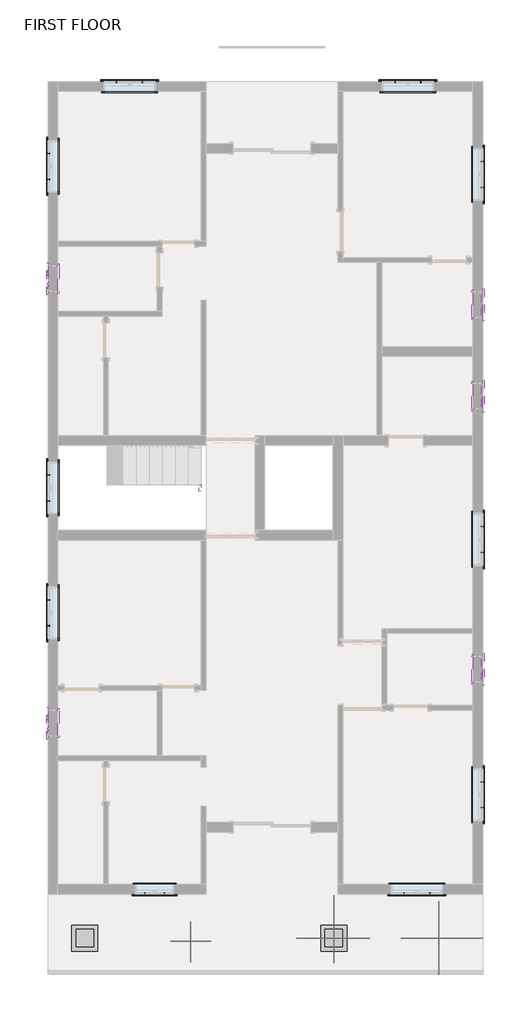
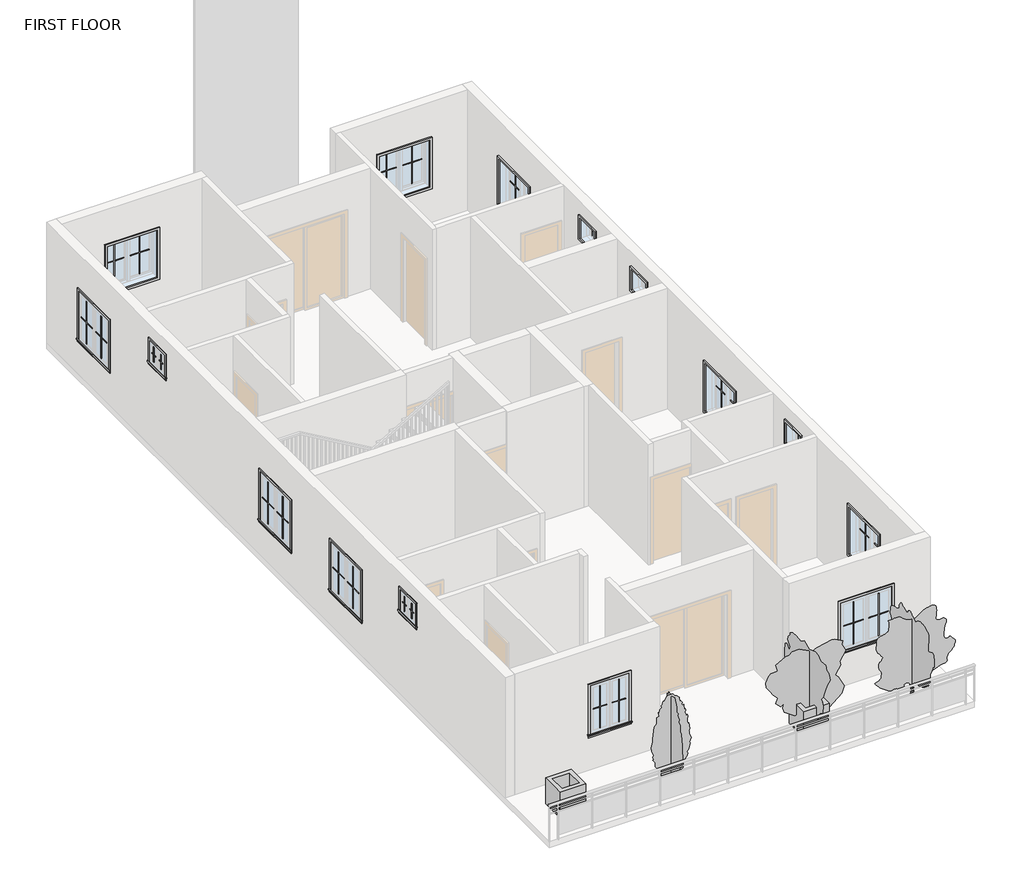
# One storey, part 4 of 4: 60 proxies, 5 geographic elements, 1 railing.
"""IFC4 building model written with IfcOpenShell, lengths in millimetres."""

from ifc_helpers import new_model, si_unit, frame, origin, place, context, project, spatial, polyline, outline, extrude, transform, mapped, element, save
from components import muntin_pattern_2x2_muntin_pattern_2x2_4dfeb3f3, muntin_pattern_2x2_muntin_pattern_2x2_e852a7e4, muntin_pattern_2x2_muntin_pattern_2x2_1acec82f, muntin_pattern_2x2_muntin_pattern_2x2_43d02eee, muntin_pattern_2x2_muntin_pattern_2x2_653c8599, muntin_pattern_2x2_muntin_pattern_2x2_c179cf80, trim_window_exterior_flat_with_sill_7cfdd449, trim_window_exterior_flat_with_sill_e4b28ec3, trim_window_exterior_flat_with_sill_e6f34eb5, trim_window_interior_flat_picture_frame_f1e0b15b, trim_window_interior_flat_picture_frame_39ff4276, trim_window_interior_flat_picture_frame_9a74d23d, planter_2_x2_5b049b04, rpc_tree_conifer_chinese_juniper_7_2_1b9786cd, rpc_tree_fall_american_beech_20_7ed35302, rpc_tree_fall_service_berry_25_c2e4521a

model = new_model("IFC4")

# Units and contexts
model_context = context("Model", 3, world=origin())
ifc_project = project(units=[si_unit("LENGTHUNIT", "METRE", prefix="MILLI")], contexts=[model_context])

# Site, building, storey
site = spatial("IfcSite", under=ifc_project)
building = spatial("IfcBuilding", under=site)
storey = spatial("IfcBuildingStorey", under=building, Name="FIRST FLOOR", Elevation=3200.4)

# Proxies
placement = place(None, origin())
muntin_pattern_2x2_muntin_pattern_2x2_shape = muntin_pattern_2x2_muntin_pattern_2x2_4dfeb3f3(model_context)
element("IfcBuildingElementProxy", 1, Name="Muntin Pattern_2x2 : Muntin Pattern_2x2", ObjectType="Muntin Pattern_2x2 : Muntin Pattern_2x2", at=placement, inside=storey, context=model_context, shape_type="MappedRepresentation", body=[
    mapped(muntin_pattern_2x2_muntin_pattern_2x2_shape, transform((-4756.4414041, 10049.2903263, 4184.65), x_axis=(1.0, 0.0, 0.0), y_axis=(0.0, 1.0, 0.0), z_axis=(0.0, 0.0, 1.0))),
])
element("IfcBuildingElementProxy", 2, Name="Muntin Pattern_2x2 : Muntin Pattern_2x2", ObjectType="Muntin Pattern_2x2 : Muntin Pattern_2x2", at=placement, inside=storey, context=model_context, shape_type="MappedRepresentation", body=[
    mapped(muntin_pattern_2x2_muntin_pattern_2x2_shape, transform((-6348.7039041, 7774.4028263, 4184.65), x_axis=(0.0, 1.0, 0.0), y_axis=(-1.0, 0.0, 0.0), z_axis=(0.0, 0.0, 1.0))),
])
element("IfcBuildingElementProxy", 3, Name="Muntin Pattern_2x2 : Muntin Pattern_2x2", ObjectType="Muntin Pattern_2x2 : Muntin Pattern_2x2", at=placement, inside=storey, context=model_context, shape_type="MappedRepresentation", body=[
    mapped(muntin_pattern_2x2_muntin_pattern_2x2_shape, transform((-6348.7039041, -2664.9971737, 4184.65), x_axis=(0.0, 1.0, 0.0), y_axis=(-1.0, 0.0, 0.0), z_axis=(0.0, 0.0, 1.0))),
])
element("IfcBuildingElementProxy", 4, Name="Muntin Pattern_2x2 : Muntin Pattern_2x2", ObjectType="Muntin Pattern_2x2 : Muntin Pattern_2x2", at=placement, inside=storey, context=model_context, shape_type="MappedRepresentation", body=[
    mapped(muntin_pattern_2x2_muntin_pattern_2x2_shape, transform((2575.0232801, -8930.8596737, 4184.65), x_axis=(-1.0, 0.0, 0.0), y_axis=(0.0, -1.0, 0.0), z_axis=(0.0, 0.0, 1.0))),
])
element("IfcBuildingElementProxy", 5, Name="Muntin Pattern_2x2 : Muntin Pattern_2x2", ObjectType="Muntin Pattern_2x2 : Muntin Pattern_2x2", at=placement, inside=storey, context=model_context, shape_type="MappedRepresentation", body=[
    mapped(muntin_pattern_2x2_muntin_pattern_2x2_shape, transform((3804.9460959, -6313.0721737, 4184.65), x_axis=(0.0, -1.0, 0.0), y_axis=(1.0, 0.0, 0.0), z_axis=(0.0, 0.0, 1.0))),
])
element("IfcBuildingElementProxy", 6, Name="Muntin Pattern_2x2 : Muntin Pattern_2x2", ObjectType="Muntin Pattern_2x2 : Muntin Pattern_2x2", at=placement, inside=storey, context=model_context, shape_type="MappedRepresentation", body=[
    mapped(muntin_pattern_2x2_muntin_pattern_2x2_shape, transform((3804.9460959, -344.0721737, 4184.65), x_axis=(0.0, -1.0, 0.0), y_axis=(1.0, 0.0, 0.0), z_axis=(0.0, 0.0, 1.0))),
])
element("IfcBuildingElementProxy", 7, Name="Muntin Pattern_2x2 : Muntin Pattern_2x2", ObjectType="Muntin Pattern_2x2 : Muntin Pattern_2x2", at=placement, inside=storey, context=model_context, shape_type="MappedRepresentation", body=[
    mapped(muntin_pattern_2x2_muntin_pattern_2x2_shape, transform((3804.9460959, 8190.3278263, 4184.65), x_axis=(0.0, -1.0, 0.0), y_axis=(1.0, 0.0, 0.0), z_axis=(0.0, 0.0, 1.0))),
])
element("IfcBuildingElementProxy", 8, Name="Muntin Pattern_2x2 : Muntin Pattern_2x2", ObjectType="Muntin Pattern_2x2 : Muntin Pattern_2x2", at=placement, inside=storey, context=model_context, shape_type="MappedRepresentation", body=[
    mapped(muntin_pattern_2x2_muntin_pattern_2x2_shape, transform((1758.6585959, 10049.2903263, 4184.65), x_axis=(1.0, 0.0, 0.0), y_axis=(0.0, 1.0, 0.0), z_axis=(0.0, 0.0, 1.0))),
])
element("IfcBuildingElementProxy", 9, Name="Muntin Pattern_2x2 : Muntin Pattern_2x2", ObjectType="Muntin Pattern_2x2 : Muntin Pattern_2x2", at=placement, inside=storey, context=model_context, shape_type="MappedRepresentation", body=[
    mapped(muntin_pattern_2x2_muntin_pattern_2x2_shape, transform((-6348.7039041, 256.0028263, 4184.65), x_axis=(0.0, 1.0, 0.0), y_axis=(-1.0, 0.0, 0.0), z_axis=(0.0, 0.0, 1.0))),
])
muntin_pattern_2x2_muntin_pattern_2x2_2_shape = muntin_pattern_2x2_muntin_pattern_2x2_e852a7e4(model_context)
element("IfcBuildingElementProxy", 10, Name="Muntin Pattern_2x2 : Muntin Pattern_2x2", ObjectType="Muntin Pattern_2x2 : Muntin Pattern_2x2", at=placement, inside=storey, context=model_context, shape_type="MappedRepresentation", body=[
    mapped(muntin_pattern_2x2_muntin_pattern_2x2_2_shape, transform((-4150.0164041, 10049.2903263, 4184.65), x_axis=(-1.0, 0.0, 0.0), y_axis=(0.0, -1.0, 0.0), z_axis=(0.0, 0.0, 1.0))),
])
element("IfcBuildingElementProxy", 11, Name="Muntin Pattern_2x2 : Muntin Pattern_2x2", ObjectType="Muntin Pattern_2x2 : Muntin Pattern_2x2", at=placement, inside=storey, context=model_context, shape_type="MappedRepresentation", body=[
    mapped(muntin_pattern_2x2_muntin_pattern_2x2_2_shape, transform((-6348.7039041, 8380.8278263, 4184.65), x_axis=(0.0, -1.0, 0.0), y_axis=(1.0, 0.0, 0.0), z_axis=(0.0, 0.0, 1.0))),
])
element("IfcBuildingElementProxy", 12, Name="Muntin Pattern_2x2 : Muntin Pattern_2x2", ObjectType="Muntin Pattern_2x2 : Muntin Pattern_2x2", at=placement, inside=storey, context=model_context, shape_type="MappedRepresentation", body=[
    mapped(muntin_pattern_2x2_muntin_pattern_2x2_2_shape, transform((-6348.7039041, -2058.5721737, 4184.65), x_axis=(0.0, -1.0, 0.0), y_axis=(1.0, 0.0, 0.0), z_axis=(0.0, 0.0, 1.0))),
])
element("IfcBuildingElementProxy", 13, Name="Muntin Pattern_2x2 : Muntin Pattern_2x2", ObjectType="Muntin Pattern_2x2 : Muntin Pattern_2x2", at=placement, inside=storey, context=model_context, shape_type="MappedRepresentation", body=[
    mapped(muntin_pattern_2x2_muntin_pattern_2x2_2_shape, transform((1968.5982801, -8930.8596737, 4184.65), x_axis=(1.0, 0.0, 0.0), y_axis=(0.0, 1.0, 0.0), z_axis=(0.0, 0.0, 1.0))),
])
element("IfcBuildingElementProxy", 14, Name="Muntin Pattern_2x2 : Muntin Pattern_2x2", ObjectType="Muntin Pattern_2x2 : Muntin Pattern_2x2", at=placement, inside=storey, context=model_context, shape_type="MappedRepresentation", body=[
    mapped(muntin_pattern_2x2_muntin_pattern_2x2_2_shape, transform((3804.9460959, -6919.4971737, 4184.65), x_axis=(0.0, 1.0, 0.0), y_axis=(-1.0, 0.0, 0.0), z_axis=(0.0, 0.0, 1.0))),
])
element("IfcBuildingElementProxy", 15, Name="Muntin Pattern_2x2 : Muntin Pattern_2x2", ObjectType="Muntin Pattern_2x2 : Muntin Pattern_2x2", at=placement, inside=storey, context=model_context, shape_type="MappedRepresentation", body=[
    mapped(muntin_pattern_2x2_muntin_pattern_2x2_2_shape, transform((3804.9460959, -950.4971737, 4184.65), x_axis=(0.0, 1.0, 0.0), y_axis=(-1.0, 0.0, 0.0), z_axis=(0.0, 0.0, 1.0))),
])
element("IfcBuildingElementProxy", 16, Name="Muntin Pattern_2x2 : Muntin Pattern_2x2", ObjectType="Muntin Pattern_2x2 : Muntin Pattern_2x2", at=placement, inside=storey, context=model_context, shape_type="MappedRepresentation", body=[
    mapped(muntin_pattern_2x2_muntin_pattern_2x2_2_shape, transform((3804.9460959, 7583.9028263, 4184.65), x_axis=(0.0, 1.0, 0.0), y_axis=(-1.0, 0.0, 0.0), z_axis=(0.0, 0.0, 1.0))),
])
element("IfcBuildingElementProxy", 17, Name="Muntin Pattern_2x2 : Muntin Pattern_2x2", ObjectType="Muntin Pattern_2x2 : Muntin Pattern_2x2", at=placement, inside=storey, context=model_context, shape_type="MappedRepresentation", body=[
    mapped(muntin_pattern_2x2_muntin_pattern_2x2_2_shape, transform((2365.0835959, 10049.2903263, 4184.65), x_axis=(-1.0, 0.0, 0.0), y_axis=(0.0, -1.0, 0.0), z_axis=(0.0, 0.0, 1.0))),
])
element("IfcBuildingElementProxy", 18, Name="Muntin Pattern_2x2 : Muntin Pattern_2x2", ObjectType="Muntin Pattern_2x2 : Muntin Pattern_2x2", at=placement, inside=storey, context=model_context, shape_type="MappedRepresentation", body=[
    mapped(muntin_pattern_2x2_muntin_pattern_2x2_2_shape, transform((-6348.7039041, 862.4278263, 4184.65), x_axis=(0.0, -1.0, 0.0), y_axis=(1.0, 0.0, 0.0), z_axis=(0.0, 0.0, 1.0))),
])
muntin_pattern_2x2_muntin_pattern_2x2_3_shape = muntin_pattern_2x2_muntin_pattern_2x2_1acec82f(model_context)
element("IfcBuildingElementProxy", 19, Name="Muntin Pattern_2x2 : Muntin Pattern_2x2", ObjectType="Muntin Pattern_2x2 : Muntin Pattern_2x2", at=placement, inside=storey, context=model_context, shape_type="MappedRepresentation", body=[
    mapped(muntin_pattern_2x2_muntin_pattern_2x2_3_shape, transform((-3635.6664041, -8930.8596737, 4184.65), x_axis=(-1.0, 0.0, 0.0), y_axis=(0.0, -1.0, 0.0), z_axis=(0.0, 0.0, 1.0))),
])
muntin_pattern_2x2_muntin_pattern_2x2_4_shape = muntin_pattern_2x2_muntin_pattern_2x2_43d02eee(model_context)
element("IfcBuildingElementProxy", 20, Name="Muntin Pattern_2x2 : Muntin Pattern_2x2", ObjectType="Muntin Pattern_2x2 : Muntin Pattern_2x2", at=placement, inside=storey, context=model_context, shape_type="MappedRepresentation", body=[
    mapped(muntin_pattern_2x2_muntin_pattern_2x2_4_shape, transform((-4089.6914041, -8930.8596737, 4184.65), x_axis=(1.0, 0.0, 0.0), y_axis=(0.0, 1.0, 0.0), z_axis=(0.0, 0.0, 1.0))),
])
muntin_pattern_2x2_muntin_pattern_2x2_5_shape = muntin_pattern_2x2_muntin_pattern_2x2_653c8599(model_context)
element("IfcBuildingElementProxy", 21, Name="Muntin Pattern_2x2 : Muntin Pattern_2x2", ObjectType="Muntin Pattern_2x2 : Muntin Pattern_2x2", at=placement, inside=storey, context=model_context, shape_type="MappedRepresentation", body=[
    mapped(muntin_pattern_2x2_muntin_pattern_2x2_5_shape, transform((-6348.7039041, 5297.9028263, 5403.85), x_axis=(0.0, 1.0, 0.0), y_axis=(-1.0, 0.0, 0.0), z_axis=(0.0, 0.0, 1.0))),
])
element("IfcBuildingElementProxy", 22, Name="Muntin Pattern_2x2 : Muntin Pattern_2x2", ObjectType="Muntin Pattern_2x2 : Muntin Pattern_2x2", at=placement, inside=storey, context=model_context, shape_type="MappedRepresentation", body=[
    mapped(muntin_pattern_2x2_muntin_pattern_2x2_5_shape, transform((-6348.7039041, -5090.6971737, 5403.85), x_axis=(0.0, 1.0, 0.0), y_axis=(-1.0, 0.0, 0.0), z_axis=(0.0, 0.0, 1.0))),
])
element("IfcBuildingElementProxy", 23, Name="Muntin Pattern_2x2 : Muntin Pattern_2x2", ObjectType="Muntin Pattern_2x2 : Muntin Pattern_2x2", at=placement, inside=storey, context=model_context, shape_type="MappedRepresentation", body=[
    mapped(muntin_pattern_2x2_muntin_pattern_2x2_5_shape, transform((3804.9460959, -3531.7721737, 5403.85), x_axis=(0.0, -1.0, 0.0), y_axis=(1.0, 0.0, 0.0), z_axis=(0.0, 0.0, 1.0))),
])
element("IfcBuildingElementProxy", 24, Name="Muntin Pattern_2x2 : Muntin Pattern_2x2", ObjectType="Muntin Pattern_2x2 : Muntin Pattern_2x2", at=placement, inside=storey, context=model_context, shape_type="MappedRepresentation", body=[
    mapped(muntin_pattern_2x2_muntin_pattern_2x2_5_shape, transform((3804.9460959, 2856.3278263, 5403.85), x_axis=(0.0, -1.0, 0.0), y_axis=(1.0, 0.0, 0.0), z_axis=(0.0, 0.0, 1.0))),
])
element("IfcBuildingElementProxy", 25, Name="Muntin Pattern_2x2 : Muntin Pattern_2x2", ObjectType="Muntin Pattern_2x2 : Muntin Pattern_2x2", at=placement, inside=storey, context=model_context, shape_type="MappedRepresentation", body=[
    mapped(muntin_pattern_2x2_muntin_pattern_2x2_5_shape, transform((3804.9460959, 4996.2778263, 5403.85), x_axis=(0.0, -1.0, 0.0), y_axis=(1.0, 0.0, 0.0), z_axis=(0.0, 0.0, 1.0))),
])
muntin_pattern_2x2_muntin_pattern_2x2_6_shape = muntin_pattern_2x2_muntin_pattern_2x2_c179cf80(model_context)
element("IfcBuildingElementProxy", 26, Name="Muntin Pattern_2x2 : Muntin Pattern_2x2", ObjectType="Muntin Pattern_2x2 : Muntin Pattern_2x2", at=placement, inside=storey, context=model_context, shape_type="MappedRepresentation", body=[
    mapped(muntin_pattern_2x2_muntin_pattern_2x2_6_shape, transform((-6348.7039041, 5599.5278263, 5403.85), x_axis=(0.0, -1.0, 0.0), y_axis=(1.0, 0.0, 0.0), z_axis=(0.0, 0.0, 1.0))),
])
element("IfcBuildingElementProxy", 27, Name="Muntin Pattern_2x2 : Muntin Pattern_2x2", ObjectType="Muntin Pattern_2x2 : Muntin Pattern_2x2", at=placement, inside=storey, context=model_context, shape_type="MappedRepresentation", body=[
    mapped(muntin_pattern_2x2_muntin_pattern_2x2_6_shape, transform((-6348.7039041, -4789.0721737, 5403.85), x_axis=(0.0, -1.0, 0.0), y_axis=(1.0, 0.0, 0.0), z_axis=(0.0, 0.0, 1.0))),
])
element("IfcBuildingElementProxy", 28, Name="Muntin Pattern_2x2 : Muntin Pattern_2x2", ObjectType="Muntin Pattern_2x2 : Muntin Pattern_2x2", at=placement, inside=storey, context=model_context, shape_type="MappedRepresentation", body=[
    mapped(muntin_pattern_2x2_muntin_pattern_2x2_6_shape, transform((3804.9460959, -3833.3971737, 5403.85), x_axis=(0.0, 1.0, 0.0), y_axis=(-1.0, 0.0, 0.0), z_axis=(0.0, 0.0, 1.0))),
])
element("IfcBuildingElementProxy", 29, Name="Muntin Pattern_2x2 : Muntin Pattern_2x2", ObjectType="Muntin Pattern_2x2 : Muntin Pattern_2x2", at=placement, inside=storey, context=model_context, shape_type="MappedRepresentation", body=[
    mapped(muntin_pattern_2x2_muntin_pattern_2x2_6_shape, transform((3804.9460959, 2554.7028263, 5403.85), x_axis=(0.0, 1.0, 0.0), y_axis=(-1.0, 0.0, 0.0), z_axis=(0.0, 0.0, 1.0))),
])
element("IfcBuildingElementProxy", 30, Name="Muntin Pattern_2x2 : Muntin Pattern_2x2", ObjectType="Muntin Pattern_2x2 : Muntin Pattern_2x2", at=placement, inside=storey, context=model_context, shape_type="MappedRepresentation", body=[
    mapped(muntin_pattern_2x2_muntin_pattern_2x2_6_shape, transform((3804.9460959, 4694.6528263, 5403.85), x_axis=(0.0, 1.0, 0.0), y_axis=(-1.0, 0.0, 0.0), z_axis=(0.0, 0.0, 1.0))),
])
trim_window_exterior_flat_with_sill_shape = trim_window_exterior_flat_with_sill_7cfdd449(model_context)
element("IfcBuildingElementProxy", 31, Name="Trim-Window-Exterior-Flat : with Sill", ObjectType="Trim-Window-Exterior-Flat : with Sill", at=placement, inside=storey, context=model_context, shape_type="MappedRepresentation", body=[
    mapped(trim_window_exterior_flat_with_sill_shape, transform((-4453.2289041, 10058.8153263, 5334.0), x_axis=(-1.0, 0.0, 0.0), y_axis=(0.0, 0.0, 1.0), z_axis=(0.0, 1.0, 0.0))),
])
element("IfcBuildingElementProxy", 32, Name="Trim-Window-Exterior-Flat : with Sill", ObjectType="Trim-Window-Exterior-Flat : with Sill", at=placement, inside=storey, context=model_context, shape_type="MappedRepresentation", body=[
    mapped(trim_window_exterior_flat_with_sill_shape, transform((-6358.2289041, 8077.6153263, 5334.0), x_axis=(0.0, -1.0, 0.0), y_axis=(0.0, 0.0, 1.0), z_axis=(-1.0, 0.0, 0.0))),
])
element("IfcBuildingElementProxy", 33, Name="Trim-Window-Exterior-Flat : with Sill", ObjectType="Trim-Window-Exterior-Flat : with Sill", at=placement, inside=storey, context=model_context, shape_type="MappedRepresentation", body=[
    mapped(trim_window_exterior_flat_with_sill_shape, transform((-6358.2289041, -2361.7846737, 5334.0), x_axis=(0.0, -1.0, 0.0), y_axis=(0.0, 0.0, 1.0), z_axis=(-1.0, 0.0, 0.0))),
])
element("IfcBuildingElementProxy", 34, Name="Trim-Window-Exterior-Flat : with Sill", ObjectType="Trim-Window-Exterior-Flat : with Sill", at=placement, inside=storey, context=model_context, shape_type="MappedRepresentation", body=[
    mapped(trim_window_exterior_flat_with_sill_shape, transform((2271.8107801, -8940.3846737, 5334.0), x_axis=(1.0, 0.0, 0.0), y_axis=(0.0, 0.0, 1.0), z_axis=(0.0, -1.0, 0.0))),
])
element("IfcBuildingElementProxy", 35, Name="Trim-Window-Exterior-Flat : with Sill", ObjectType="Trim-Window-Exterior-Flat : with Sill", at=placement, inside=storey, context=model_context, shape_type="MappedRepresentation", body=[
    mapped(trim_window_exterior_flat_with_sill_shape, transform((3814.4710959, -6616.2846737, 5334.0), x_axis=(0.0, 1.0, 0.0), y_axis=(0.0, 0.0, 1.0), z_axis=(1.0, 0.0, 0.0))),
])
element("IfcBuildingElementProxy", 36, Name="Trim-Window-Exterior-Flat : with Sill", ObjectType="Trim-Window-Exterior-Flat : with Sill", at=placement, inside=storey, context=model_context, shape_type="MappedRepresentation", body=[
    mapped(trim_window_exterior_flat_with_sill_shape, transform((3814.4710959, -647.2846737, 5334.0), x_axis=(0.0, 1.0, 0.0), y_axis=(0.0, 0.0, 1.0), z_axis=(1.0, 0.0, 0.0))),
])
element("IfcBuildingElementProxy", 37, Name="Trim-Window-Exterior-Flat : with Sill", ObjectType="Trim-Window-Exterior-Flat : with Sill", at=placement, inside=storey, context=model_context, shape_type="MappedRepresentation", body=[
    mapped(trim_window_exterior_flat_with_sill_shape, transform((3814.4710959, 7887.1153263, 5334.0), x_axis=(0.0, 1.0, 0.0), y_axis=(0.0, 0.0, 1.0), z_axis=(1.0, 0.0, 0.0))),
])
element("IfcBuildingElementProxy", 38, Name="Trim-Window-Exterior-Flat : with Sill", ObjectType="Trim-Window-Exterior-Flat : with Sill", at=placement, inside=storey, context=model_context, shape_type="MappedRepresentation", body=[
    mapped(trim_window_exterior_flat_with_sill_shape, transform((2061.8710959, 10058.8153263, 5334.0), x_axis=(-1.0, 0.0, 0.0), y_axis=(0.0, 0.0, 1.0), z_axis=(0.0, 1.0, 0.0))),
])
element("IfcBuildingElementProxy", 39, Name="Trim-Window-Exterior-Flat : with Sill", ObjectType="Trim-Window-Exterior-Flat : with Sill", at=placement, inside=storey, context=model_context, shape_type="MappedRepresentation", body=[
    mapped(trim_window_exterior_flat_with_sill_shape, transform((-6358.2289041, 559.2153263, 5334.0), x_axis=(0.0, -1.0, 0.0), y_axis=(0.0, 0.0, 1.0), z_axis=(-1.0, 0.0, 0.0))),
])
trim_window_exterior_flat_with_sill_2_shape = trim_window_exterior_flat_with_sill_e4b28ec3(model_context)
element("IfcBuildingElementProxy", 40, Name="Trim-Window-Exterior-Flat : with Sill", ObjectType="Trim-Window-Exterior-Flat : with Sill", at=placement, inside=storey, context=model_context, shape_type="MappedRepresentation", body=[
    mapped(trim_window_exterior_flat_with_sill_2_shape, transform((-3862.6789041, -8940.3846737, 5334.0), x_axis=(1.0, 0.0, 0.0), y_axis=(0.0, 0.0, 1.0), z_axis=(0.0, -1.0, 0.0))),
])
trim_window_exterior_flat_with_sill_3_shape = trim_window_exterior_flat_with_sill_e6f34eb5(model_context)
element("IfcBuildingElementProxy", 41, Name="Trim-Window-Exterior-Flat : with Sill", ObjectType="Trim-Window-Exterior-Flat : with Sill", at=placement, inside=storey, context=model_context, shape_type="MappedRepresentation", body=[
    mapped(trim_window_exterior_flat_with_sill_3_shape, transform((-6358.2289041, 5448.7153263, 5867.4), x_axis=(0.0, -1.0, 0.0), y_axis=(0.0, 0.0, 1.0), z_axis=(-1.0, 0.0, 0.0))),
])
element("IfcBuildingElementProxy", 42, Name="Trim-Window-Exterior-Flat : with Sill", ObjectType="Trim-Window-Exterior-Flat : with Sill", at=placement, inside=storey, context=model_context, shape_type="MappedRepresentation", body=[
    mapped(trim_window_exterior_flat_with_sill_3_shape, transform((-6358.2289041, -4939.8846737, 5867.4), x_axis=(0.0, -1.0, 0.0), y_axis=(0.0, 0.0, 1.0), z_axis=(-1.0, 0.0, 0.0))),
])
element("IfcBuildingElementProxy", 43, Name="Trim-Window-Exterior-Flat : with Sill", ObjectType="Trim-Window-Exterior-Flat : with Sill", at=placement, inside=storey, context=model_context, shape_type="MappedRepresentation", body=[
    mapped(trim_window_exterior_flat_with_sill_3_shape, transform((3814.4710959, -3682.5846737, 5867.4), x_axis=(0.0, 1.0, 0.0), y_axis=(0.0, 0.0, 1.0), z_axis=(1.0, 0.0, 0.0))),
])
element("IfcBuildingElementProxy", 44, Name="Trim-Window-Exterior-Flat : with Sill", ObjectType="Trim-Window-Exterior-Flat : with Sill", at=placement, inside=storey, context=model_context, shape_type="MappedRepresentation", body=[
    mapped(trim_window_exterior_flat_with_sill_3_shape, transform((3814.4710959, 2705.5153263, 5867.4), x_axis=(0.0, 1.0, 0.0), y_axis=(0.0, 0.0, 1.0), z_axis=(1.0, 0.0, 0.0))),
])
element("IfcBuildingElementProxy", 45, Name="Trim-Window-Exterior-Flat : with Sill", ObjectType="Trim-Window-Exterior-Flat : with Sill", at=placement, inside=storey, context=model_context, shape_type="MappedRepresentation", body=[
    mapped(trim_window_exterior_flat_with_sill_3_shape, transform((3814.4710959, 4845.4653263, 5867.4), x_axis=(0.0, 1.0, 0.0), y_axis=(0.0, 0.0, 1.0), z_axis=(1.0, 0.0, 0.0))),
])
trim_window_interior_flat_picture_frame_shape = trim_window_interior_flat_picture_frame_f1e0b15b(model_context)
element("IfcBuildingElementProxy", 46, Name="Trim-Window-Interior-Flat : Picture Frame", ObjectType="Trim-Window-Interior-Flat : Picture Frame", at=placement, inside=storey, context=model_context, shape_type="MappedRepresentation", body=[
    mapped(trim_window_interior_flat_picture_frame_shape, transform((-4453.2289041, 9830.2153263, 5334.0), x_axis=(1.0, 0.0, 0.0), y_axis=(0.0, 0.0, 1.0), z_axis=(0.0, -1.0, 0.0))),
])
element("IfcBuildingElementProxy", 47, Name="Trim-Window-Interior-Flat : Picture Frame", ObjectType="Trim-Window-Interior-Flat : Picture Frame", at=placement, inside=storey, context=model_context, shape_type="MappedRepresentation", body=[
    mapped(trim_window_interior_flat_picture_frame_shape, transform((-6129.6289041, 8077.6153263, 5334.0), x_axis=(0.0, 1.0, 0.0), y_axis=(0.0, 0.0, 1.0), z_axis=(1.0, 0.0, 0.0))),
])
element("IfcBuildingElementProxy", 48, Name="Trim-Window-Interior-Flat : Picture Frame", ObjectType="Trim-Window-Interior-Flat : Picture Frame", at=placement, inside=storey, context=model_context, shape_type="MappedRepresentation", body=[
    mapped(trim_window_interior_flat_picture_frame_shape, transform((-6129.6289041, -2361.7846737, 5334.0), x_axis=(0.0, 1.0, 0.0), y_axis=(0.0, 0.0, 1.0), z_axis=(1.0, 0.0, 0.0))),
])
element("IfcBuildingElementProxy", 49, Name="Trim-Window-Interior-Flat : Picture Frame", ObjectType="Trim-Window-Interior-Flat : Picture Frame", at=placement, inside=storey, context=model_context, shape_type="MappedRepresentation", body=[
    mapped(trim_window_interior_flat_picture_frame_shape, transform((2271.8107801, -8711.7846737, 5334.0), x_axis=(-1.0, 0.0, 0.0), y_axis=(0.0, 0.0, 1.0), z_axis=(0.0, 1.0, 0.0))),
])
element("IfcBuildingElementProxy", 50, Name="Trim-Window-Interior-Flat : Picture Frame", ObjectType="Trim-Window-Interior-Flat : Picture Frame", at=placement, inside=storey, context=model_context, shape_type="MappedRepresentation", body=[
    mapped(trim_window_interior_flat_picture_frame_shape, transform((3585.8710959, -6616.2846737, 5334.0), x_axis=(0.0, -1.0, 0.0), y_axis=(0.0, 0.0, 1.0), z_axis=(-1.0, 0.0, 0.0))),
])
element("IfcBuildingElementProxy", 51, Name="Trim-Window-Interior-Flat : Picture Frame", ObjectType="Trim-Window-Interior-Flat : Picture Frame", at=placement, inside=storey, context=model_context, shape_type="MappedRepresentation", body=[
    mapped(trim_window_interior_flat_picture_frame_shape, transform((3585.8710959, -647.2846737, 5334.0), x_axis=(0.0, -1.0, 0.0), y_axis=(0.0, 0.0, 1.0), z_axis=(-1.0, 0.0, 0.0))),
])
element("IfcBuildingElementProxy", 52, Name="Trim-Window-Interior-Flat : Picture Frame", ObjectType="Trim-Window-Interior-Flat : Picture Frame", at=placement, inside=storey, context=model_context, shape_type="MappedRepresentation", body=[
    mapped(trim_window_interior_flat_picture_frame_shape, transform((3585.8710959, 7887.1153263, 5334.0), x_axis=(0.0, -1.0, 0.0), y_axis=(0.0, 0.0, 1.0), z_axis=(-1.0, 0.0, 0.0))),
])
element("IfcBuildingElementProxy", 53, Name="Trim-Window-Interior-Flat : Picture Frame", ObjectType="Trim-Window-Interior-Flat : Picture Frame", at=placement, inside=storey, context=model_context, shape_type="MappedRepresentation", body=[
    mapped(trim_window_interior_flat_picture_frame_shape, transform((2061.8710959, 9830.2153263, 5334.0), x_axis=(1.0, 0.0, 0.0), y_axis=(0.0, 0.0, 1.0), z_axis=(0.0, -1.0, 0.0))),
])
element("IfcBuildingElementProxy", 54, Name="Trim-Window-Interior-Flat : Picture Frame", ObjectType="Trim-Window-Interior-Flat : Picture Frame", at=placement, inside=storey, context=model_context, shape_type="MappedRepresentation", body=[
    mapped(trim_window_interior_flat_picture_frame_shape, transform((-6129.6289041, 559.2153263, 5334.0), x_axis=(0.0, 1.0, 0.0), y_axis=(0.0, 0.0, 1.0), z_axis=(1.0, 0.0, 0.0))),
])
trim_window_interior_flat_picture_frame_2_shape = trim_window_interior_flat_picture_frame_39ff4276(model_context)
element("IfcBuildingElementProxy", 55, Name="Trim-Window-Interior-Flat : Picture Frame", ObjectType="Trim-Window-Interior-Flat : Picture Frame", at=placement, inside=storey, context=model_context, shape_type="MappedRepresentation", body=[
    mapped(trim_window_interior_flat_picture_frame_2_shape, transform((-3862.6789041, -8711.7846737, 5334.0), x_axis=(-1.0, 0.0, 0.0), y_axis=(0.0, 0.0, 1.0), z_axis=(0.0, 1.0, 0.0))),
])
trim_window_interior_flat_picture_frame_3_shape = trim_window_interior_flat_picture_frame_9a74d23d(model_context)
element("IfcBuildingElementProxy", 56, Name="Trim-Window-Interior-Flat : Picture Frame", ObjectType="Trim-Window-Interior-Flat : Picture Frame", at=placement, inside=storey, context=model_context, shape_type="MappedRepresentation", body=[
    mapped(trim_window_interior_flat_picture_frame_3_shape, transform((-6129.6289041, 5448.7153263, 5867.4), x_axis=(0.0, 1.0, 0.0), y_axis=(0.0, 0.0, 1.0), z_axis=(1.0, 0.0, 0.0))),
])
element("IfcBuildingElementProxy", 57, Name="Trim-Window-Interior-Flat : Picture Frame", ObjectType="Trim-Window-Interior-Flat : Picture Frame", at=placement, inside=storey, context=model_context, shape_type="MappedRepresentation", body=[
    mapped(trim_window_interior_flat_picture_frame_3_shape, transform((-6129.6289041, -4939.8846737, 5867.4), x_axis=(0.0, 1.0, 0.0), y_axis=(0.0, 0.0, 1.0), z_axis=(1.0, 0.0, 0.0))),
])
element("IfcBuildingElementProxy", 58, Name="Trim-Window-Interior-Flat : Picture Frame", ObjectType="Trim-Window-Interior-Flat : Picture Frame", at=placement, inside=storey, context=model_context, shape_type="MappedRepresentation", body=[
    mapped(trim_window_interior_flat_picture_frame_3_shape, transform((3585.8710959, -3682.5846737, 5867.4), x_axis=(0.0, -1.0, 0.0), y_axis=(0.0, 0.0, 1.0), z_axis=(-1.0, 0.0, 0.0))),
])
element("IfcBuildingElementProxy", 59, Name="Trim-Window-Interior-Flat : Picture Frame", ObjectType="Trim-Window-Interior-Flat : Picture Frame", at=placement, inside=storey, context=model_context, shape_type="MappedRepresentation", body=[
    mapped(trim_window_interior_flat_picture_frame_3_shape, transform((3585.8710959, 2705.5153263, 5867.4), x_axis=(0.0, -1.0, 0.0), y_axis=(0.0, 0.0, 1.0), z_axis=(-1.0, 0.0, 0.0))),
])
element("IfcBuildingElementProxy", 60, Name="Trim-Window-Interior-Flat : Picture Frame", ObjectType="Trim-Window-Interior-Flat : Picture Frame", at=placement, inside=storey, context=model_context, shape_type="MappedRepresentation", body=[
    mapped(trim_window_interior_flat_picture_frame_3_shape, transform((3585.8710959, 4845.4653263, 5867.4), x_axis=(0.0, -1.0, 0.0), y_axis=(0.0, 0.0, 1.0), z_axis=(-1.0, 0.0, 0.0))),
])

# Geographic elements
planter_2_x2_shape = planter_2_x2_5b049b04(model_context)
element("IfcGeographicElement", 61, ObjectType="Planter : 2'X2'", at=placement, inside=storey, context=model_context, shape_type="MappedRepresentation", body=[
    mapped(planter_2_x2_shape, transform((-5500.9789041, -9969.0846737, 3200.4), x_axis=(1.0, 0.0, 0.0), y_axis=(0.0, 1.0, 0.0), z_axis=(0.0, 0.0, 1.0))),
])
element("IfcGeographicElement", 62, ObjectType="Planter : 2'X2'", at=placement, inside=storey, context=model_context, shape_type="MappedRepresentation", body=[
    mapped(planter_2_x2_shape, transform((328.3210959, -9969.0846737, 3200.4), x_axis=(1.0, 0.0, 0.0), y_axis=(0.0, 1.0, 0.0), z_axis=(0.0, 0.0, 1.0))),
])
rpc_tree_conifer_chinese_juniper_7_2_shape = rpc_tree_conifer_chinese_juniper_7_2_1b9786cd(model_context)
element("IfcGeographicElement", 63, ObjectType="RPC Tree - Conifer : Chinese Juniper - 7' 2", at=placement, inside=storey, context=model_context, shape_type="MappedRepresentation", body=[
    mapped(rpc_tree_conifer_chinese_juniper_7_2_shape, transform((-3024.6755752, -10045.2846737, 3200.4), x_axis=(1.0, 0.0, 0.0), y_axis=(0.0, 1.0, 0.0), z_axis=(0.0, 0.0, 1.0))),
])
rpc_tree_fall_american_beech_20_shape = rpc_tree_fall_american_beech_20_7ed35302(model_context)
element("IfcGeographicElement", 64, ObjectType="RPC Tree - Fall : American Beech - 20'", at=placement, inside=storey, context=model_context, shape_type="MappedRepresentation", body=[
    mapped(rpc_tree_fall_american_beech_20_shape, transform((2785.7710959, -9969.0846737, 3200.4), x_axis=(1.0, 0.0, 0.0), y_axis=(0.0, 1.0, 0.0), z_axis=(0.0, 0.0, 1.0))),
])
rpc_tree_fall_service_berry_25_shape = rpc_tree_fall_service_berry_25_c2e4521a(model_context)
element("IfcGeographicElement", 65, ObjectType="RPC Tree - Fall : Service Berry - 25'", at=placement, inside=storey, context=model_context, shape_type="MappedRepresentation", body=[
    mapped(rpc_tree_fall_service_berry_25_shape, transform((328.3210959, -9969.0846737, 3200.4), x_axis=(1.0, 0.0, 0.0), y_axis=(0.0, 1.0, 0.0), z_axis=(0.0, 0.0, 1.0))),
])

# Railing
element("IfcRailing", 66, ObjectType="Handrail - Rectangular", at=placement, inside=storey, context=model_context, shape_type="SweptSolid", body=[
    extrude(outline(polyline([(-2827.6289041, 635.4153263), (-2776.8289041, 635.4153263), (-2776.8289041, 483.0153263), (-2827.6289041, 483.0153263), (-2827.6289041, 635.4153263)])), frame((0.0, 0.0, 5664.2), z_axis=(0.0, 0.0, 1.0), x_axis=(1.0, 0.0, 0.0)), (0.0, 0.0, 1.0), 50.8),
    extrude(outline(polyline([(-2792.7039041, 543.3403263), (-2792.7039041, 524.2903263), (-2811.7539041, 524.2903263), (-2811.7539041, 543.3403263), (-2792.7039041, 543.3403263)])), frame((0.0, 0.0, 4800.6), z_axis=(0.0, 0.0, 1.0), x_axis=(1.0, 0.0, 0.0)), (0.0, 0.0, 1.0), 863.6),
    extrude(outline(polyline([(-2792.7039041, 502.0653263), (-2792.7039041, 483.0153263), (-2811.7539041, 483.0153263), (-2811.7539041, 502.0653263), (-2792.7039041, 502.0653263)])), frame((0.0, 0.0, 4800.6), z_axis=(0.0, 0.0, 1.0), x_axis=(1.0, 0.0, 0.0)), (0.0, 0.0, 1.0), 863.6),
    extrude(outline(polyline([(-2792.7039041, 635.4153263), (-2792.7039041, 616.3653263), (-2811.7539041, 616.3653263), (-2811.7539041, 635.4153263), (-2792.7039041, 635.4153263)])), frame((0.0, 0.0, 4800.6), z_axis=(0.0, 0.0, 1.0), x_axis=(1.0, 0.0, 0.0)), (0.0, 0.0, 1.0), 863.6),
])

save(model, "model.ifc")

# Revit data of these elements
# Type "Muntin Pattern_2x2 : Muntin Pattern_2x2"
#   Width [instance default] = 4' - 0"
#   Thickness = 0' - 0 1/2"
#   Height [instance default] = 4' - 0"
#   Distance = 0' - 0 3/4"
#   Interior Material [instance default] = none
#   Exterior Material [instance default] = none
#   Default Elevation = 0
# Type "Trim-Window-Exterior-Flat : with Sill"
#   Trim Width = 0' - 2 1/4"
#   Trim Thickness_Picture Frame = 0' - 1 1/4"
#   Trim Thickness_with Sill = 0' - 0 3/4"
#   Sill Thickness = 0' - 1 1/4"
#   Opening Width [instance default] = 2' - 0"
#   Opening Height [instance default] = 3' - 0"
#   Default Elevation = 4' - 0"
#   Sill = yes
#   Picture Frame = no
#   Trim Material [instance default] = none
# Type "Trim-Window-Interior-Flat : Picture Frame"
#   Trim Thickness_Picture Frame = 0' - 1 1/4"
#   Trim Width = 0' - 2 1/4"
#   Trim Thickness_with Sill = 0' - 0 3/4"
#   Sill Thickness = 0' - 1 1/4"
#   Opening Width [instance default] = 2' - 0"
#   Opening Height [instance default] = 3' - 0"
#   Default Elevation = 4' - 0"
#   Sill = no
#   Picture Frame = yes
#   Trim Material [instance default] = none
# Type "Planter : 2'X2'"
#   Depth = 2' - 0"
#   Height = 2' - 6"
#   Width = 2' - 0"
#   Material = Concrete, Precast
# Type "RPC Tree - Conifer : Chinese Juniper - 7' 2"
#   built-in parameter 1005198 = "{2, 15},{39, RPC-16-FUM3-UUQ0-UBF0-N000-ST1L-LVER-AU},{1, 0},{1, 0},{2, 35},{1, 8},{5, Color},{1, 0},{1, 0},{3, 0.8},{3, 0.8},{3, 0.8},{1, 8},{7, BBoxMin},{1, 0},{1, 0},{1, 0},{1, 0},{1, 0},{1, 8},{7, BBoxMax},{1, 0},{1, 0},{1, 0},{1, 0},{1, 0},{2, 11},{9, RPCTypeId},{1, 0},{1, 0},{39, RPC-16-FUM3-UUQ0-UBF0-N000-ST1L-LVER-AU},{1, 6},{14, RPCPlantHeight},{1, 0},{1, 0},{1, 7},{2, 11},{7, keyword},{1, 0},{1, 0},{96, :Geometry:RPC:Chinese Juniper:juniperus chinensis:chinese:juniper:cupressaceae:conifer:evergreen},{2, 11},{8, category},{1, 0},{1, 0},{16, :Trees [General]},{2, 11},{12, LocalizedUID},{1, 0},{1, 0},{15, Chinese Juniper},{2, 14},{6, Height},{1, 0},{1, 0},{1, 7},{1, 2},{16, Cast Reflections},{1, 0},{1, 0},{1, 0},{1, 2},{12, Cast Shadows},{1, 0},{1, 0},{1, 1},{1, 2},{9, Lock View},{1, 0},{1, 0},{1, 0},{1, 4},{5, ViewC},{1, 0},{1, 0},{1, 0},{2, 11},{20, AdvancedUIDefinition},{1, 0},{1, 0},{0, },{2, 11},{10, AssetLibID},{1, 0},{1, 0},{36, 4D3F6E72-3F99-4203-98E9-AF80B3C7A7A4},{2, 11},{10, BaseSchema},{1, 0},{1, 0},{9, RPCSchema},{2, 11},{12, ExchangeGUID},{1, 0},{1, 0},{0, },{1, 2},{6, Hidden},{1, 0},{1, 0},{1, 0},{1, 4},{11, RPCCategory},{1, 0},{1, 0},{1, 0},{2, 11},{8, RPCImage},{1, 0},{1, 0},{0, },{1, 4},{13, SchemaVersion},{1, 0},{1, 0},{1, 4},{2, 11},{12, UIDefinition},{1, 0},{1, 0},{0, },{2, 11},{6, UIName},{1, 0},{1, 0},{39, RPC-16-FUM3-UUQ0-UBF0-N000-ST1L-LVER-AU},{2, 11},{11, VersionGUID},{1, 0},{1, 0},{9, RPCSchema},{2, 11},{9, assettype},{1, 0},{1, 0},{11, RPCGeometry},{2, 11},{11, description},{1, 0},{1, 0},{0, },{2, 11},{9, localname},{1, 0},{1, 0},{3, RPC},{2, 11},{9, localtype},{1, 0},{1, 0},{3, RPC},{1, 4},{8, revision},{1, 0},{1, 0},{1, 1},{2, 11},{9, thumbnail},{1, 0},{1, 0},{0, },{1, 4},{7, version},{1, 0},{1, 0},{1, 1},{1, 2},{20, RPC_Cast Reflections},{1, 0},{1, 0},{1, 1},{1, 2},{16, RPC_Cast Shadows},{1, 0},{1, 0},{1, 1},{1, 2},{13, RPC_Lock View},{1, 0},{1, 0},{1, 0},{1, 4},{9, RPC_ViewC},{1, 0},{1, 0},{1, 0},{21, assetlibrary_base.fbx},{1, 5},"
#   built-in parameter 1005195 = "RPC-16-FUM3-UUQ0-UBF0-N000-ST1L-LVER-AU"
#   Type Comments = "Chinese Juniper"
#   Assembly Code = "G2050500"
#   Height = 7' - 0"
#   Description = (empty or 0)
#   Default Elevation = 0
# Type "RPC Tree - Fall : American Beech - 20'"
#   built-in parameter 1005198 = "{2, 15},{39, RPC-16-G2VX-NFFX-5QM5-6000-ST1L-LVER-AU},{1, 0},{1, 0},{2, 13},{1, 8},{5, Color},{1, 0},{1, 0},{3, 0.8},{3, 0.8},{3, 0.8},{1, 8},{7, BBoxMin},{1, 0},{1, 0},{1, 0},{1, 0},{1, 0},{1, 8},{7, BBoxMax},{1, 0},{1, 0},{1, 0},{1, 0},{1, 0},{2, 11},{9, RPCTypeId},{1, 0},{1, 0},{39, RPC-16-G2VX-NFFX-5QM5-6000-ST1L-LVER-AU},{1, 6},{14, RPCPlantHeight},{1, 0},{1, 0},{2, 20},{2, 11},{7, keyword},{1, 0},{1, 0},{39, :RPCs:Fall Trees [General]:Geometry:RPC},{2, 11},{8, category},{1, 0},{1, 0},{20, Fall Trees [General]},{2, 11},{12, LocalizedUID},{1, 0},{1, 0},{21, American Beech [Fall]},{2, 14},{6, Height},{1, 0},{1, 0},{2, 20},{1, 2},{16, Cast Reflections},{1, 0},{1, 0},{1, 0},{1, 2},{12, Cast Shadows},{1, 0},{1, 0},{1, 1},{1, 2},{9, Lock View},{1, 0},{1, 0},{1, 0},{1, 4},{5, ViewC},{1, 0},{1, 0},{1, 0},{21, assetlibrary_base.fbx},{1, 5},"
#   built-in parameter 1005195 = "RPC-16-G2VX-NFFX-5QM5-6000-ST1L-LVER-AU"
#   Type Comments = "American Beech"
#   Assembly Code = "G2050500"
#   Height = 7' - 0"
#   Default Elevation = 0
# Type "RPC Tree - Fall : Service Berry - 25'"
#   built-in parameter 1005198 = "{2, 15},{39, RPC-16-FVGU-8VG0-7PL0-4000-ST1L-LVER-AU},{1, 0},{1, 0},{2, 13},{1, 8},{5, Color},{1, 0},{1, 0},{3, 0.8},{3, 0.8},{3, 0.8},{1, 8},{7, BBoxMin},{1, 0},{1, 0},{1, 0},{1, 0},{1, 0},{1, 8},{7, BBoxMax},{1, 0},{1, 0},{1, 0},{1, 0},{1, 0},{2, 11},{9, RPCTypeId},{1, 0},{1, 0},{39, RPC-16-FVGU-8VG0-7PL0-4000-ST1L-LVER-AU},{1, 6},{14, RPCPlantHeight},{1, 0},{1, 0},{2, 25},{2, 11},{7, keyword},{1, 0},{1, 0},{39, :RPCs:Fall Trees [General]:Geometry:RPC},{2, 11},{8, category},{1, 0},{1, 0},{20, Fall Trees [General]},{2, 11},{12, LocalizedUID},{1, 0},{1, 0},{20, Service Berry [Fall]},{2, 14},{6, Height},{1, 0},{1, 0},{2, 25},{1, 2},{16, Cast Reflections},{1, 0},{1, 0},{1, 0},{1, 2},{12, Cast Shadows},{1, 0},{1, 0},{1, 1},{1, 2},{9, Lock View},{1, 0},{1, 0},{1, 0},{1, 4},{5, ViewC},{1, 0},{1, 0},{1, 0},{21, assetlibrary_base.fbx},{1, 5},"
#   built-in parameter 1005195 = "RPC-16-FVGU-8VG0-7PL0-4000-ST1L-LVER-AU"
#   Type Comments = "Service Berry"
#   Assembly Code = "G2050500"
#   Height = 7' - 0"
#   Default Elevation = 0
# Type "Handrail - Rectangular"
#   Assembly Code = "C2010400"
#   built-in parameter 1008612 = 0.0416667 (stored number, unit not read)
#   built-in parameter 1008611 = 0.0416667 (stored number, unit not read)
#   built-in parameter 1008609 = 0.333333 (stored number, unit not read)
#   built-in parameter 1008604 = 0.166667 (stored number, unit not read)
#   built-in parameter 1008603 = 0.166667 (stored number, unit not read)
#   Railing Height = 3' - 0"
#   built-in parameter 1008630 = 2
#   built-in parameter 1008610 = 2
#   built-in parameter 1008618 = Baluster - Square : 3/4"
# Elements 1, 2, 3, 4, 5, 6, 7, 8, 9, 10, 11, 12, 13, 14, 15, 16, 17, 18 (IfcBuildingElementProxy, "Muntin Pattern_2x2 : Muntin Pattern_2x2")
#   Width = 1' - 6 5/8"
#   Height = 3' - 6 1/2"
#   Interior Material = Wood - Stained
#   Exterior Material = Clad - White
#   Phase Created = New Construction
#   Materials on its faces: "Clad - White", "Wood - Stained"
# Elements 19, 20 (IfcBuildingElementProxy, "Muntin Pattern_2x2 : Muntin Pattern_2x2")
#   Width = 1' - 0 5/8"
#   Height = 3' - 6 1/2"
#   Interior Material = Wood - Stained
#   Exterior Material = Clad - White
#   Phase Created = New Construction
#   Materials on its faces: "Clad - White", "Wood - Stained"
# Elements 21, 22, 23, 24, 25, 26, 27, 28, 29, 30 (IfcBuildingElementProxy, "Muntin Pattern_2x2 : Muntin Pattern_2x2")
#   Width = 0' - 6 5/8"
#   Height = 1' - 3 1/2"
#   Interior Material = Wood - Stained
#   Exterior Material = Clad - White
#   Phase Created = New Construction
#   Materials on its faces: "Clad - White", "Wood - Stained"
# Elements 31, 32, 33, 34, 35, 36, 37, 38, 39 (IfcBuildingElementProxy, "Trim-Window-Exterior-Flat : with Sill")
#   Opening Width = 4' - 0"
#   Opening Height = 4' - 0"
#   Trim Material = Clad - White
#   Phase Created = New Construction
#   Materials on its faces: "Clad - White"
# Element 40 (IfcBuildingElementProxy, "Trim-Window-Exterior-Flat : with Sill")
#   Opening Width = 3' - 0"
#   Opening Height = 4' - 0"
#   Trim Material = Clad - White
#   Phase Created = New Construction
#   Materials on its faces: "Clad - White"
# Elements 41, 42, 43, 44, 45 (IfcBuildingElementProxy, "Trim-Window-Exterior-Flat : with Sill")
#   Opening Width = 2' - 0"
#   Opening Height = 1' - 9"
#   Trim Material = Clad - White
#   Phase Created = New Construction
#   Materials on its faces: "Clad - White"
# Elements 46, 47, 48, 49, 50, 51, 52, 53, 54 (IfcBuildingElementProxy, "Trim-Window-Interior-Flat : Picture Frame")
#   Opening Width = 4' - 0"
#   Opening Height = 4' - 0"
#   Trim Material = Wood - Stained
#   Phase Created = New Construction
#   Materials on its faces: "Wood - Stained"
# Element 55 (IfcBuildingElementProxy, "Trim-Window-Interior-Flat : Picture Frame")
#   Opening Width = 3' - 0"
#   Opening Height = 4' - 0"
#   Trim Material = Wood - Stained
#   Phase Created = New Construction
#   Materials on its faces: "Wood - Stained"
# Elements 56, 57, 58, 59, 60 (IfcBuildingElementProxy, "Trim-Window-Interior-Flat : Picture Frame")
#   Opening Width = 2' - 0"
#   Opening Height = 1' - 9"
#   Trim Material = Wood - Stained
#   Phase Created = New Construction
#   Materials on its faces: "Wood - Stained"
# Elements 61, 62 (IfcGeographicElement, "Planter : 2'X2'")
#   Phase Created = New Construction
#   Materials on its faces: "Concrete, Precast"
# Element 63 (IfcGeographicElement, "RPC Tree - Conifer : Chinese Juniper - 7' 2")
#   Phase Created = New Construction
# Element 64 (IfcGeographicElement, "RPC Tree - Fall : American Beech - 20'")
#   Phase Created = New Construction
# Element 65 (IfcGeographicElement, "RPC Tree - Fall : Service Berry - 25'")
#   Phase Created = New Construction
# Element 66 (IfcRailing, "Handrail - Rectangular")
#   Phase Created = New Construction
# Materials
#   "Concrete, Precast": class "Concrete", colour RGB 198 187 187, transparency 0, Description = "Precast concrete", Cost = 0
#   "Clad - White": class "Wood", colour RGB 242 242 238, transparency 0, Cost = 0
#   "Wood - Stained": class "Wood", colour RGB 224 178 126, transparency 0, Cost = 0
